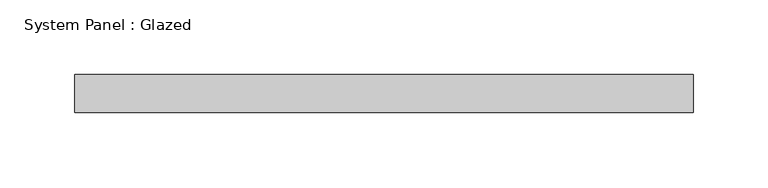
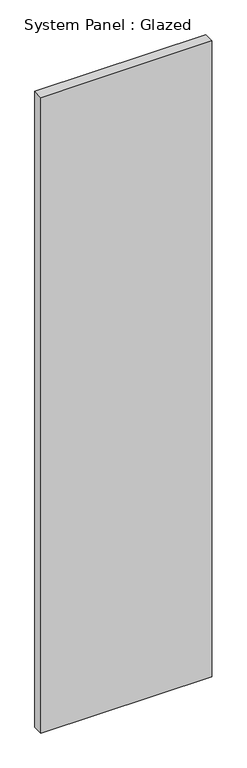
"""IFC4 building model written with IfcOpenShell, lengths in millimetres: plate geometry, System Panel : Glazed."""

from ifc_helpers import new_model, si_unit, origin, origin_with_axes, place, context, project, spatial, polyline, outline, extrude, source, transform, mapped, element, save


def system_panel_glazed_435c231b(model_context):
    return source(origin(), model_context, "Body", "SweptSolid", [
        extrude(outline(polyline([(206.375, 19.05), (-206.375, 19.05), (-206.375, 44.45), (206.375, 44.45), (206.375, 19.05)])), origin_with_axes(), (0.0, 0.0, 1.0), 1623.3622634),
    ])


if __name__ == "__main__":
    model = new_model("IFC4")
    model_context = context("Model", 3, world=origin())
    ifc_project = project(units=[si_unit("LENGTHUNIT", "METRE", prefix="MILLI")], contexts=[model_context])
    site = spatial("IfcSite", under=ifc_project)
    building = spatial("IfcBuilding", under=site)
    placement = place(None, origin())
    system_panel_glazed_shape = system_panel_glazed_435c231b(model_context)
    element("IfcPlate", 1, ObjectType="System Panel : Glazed", at=placement, inside=building, context=model_context, shape_type="MappedRepresentation", body=[
        mapped(system_panel_glazed_shape, transform((0.0, 0.0, 0.0), x_axis=(1.0, 0.0, 0.0), y_axis=(0.0, 1.0, 0.0), z_axis=(0.0, 0.0, 1.0))),
    ])
    save(model, "model.ifc")

# Revit data of these elements
# Type "System Panel : Glazed"
#   Construction Type Id = "GSP4R"
#   Analytic Construction = "1/8 in Pilkington single glazing"
#   Visual Light Transmittance = 0.9
#   Solar Heat Gain Coefficient = 0.86
#   Heat Transfer Coefficient (U) = 1.18115 BTU/(h·ft²·°F)
#   Define Thermal Properties by = 1
# Element 1 (IfcPlate, "System Panel : Glazed")
#   Materials on its faces: "Glass"
# Materials
#   "Glass": class "Glass", colour RGB 0 128 192, transparency 0.75, Description = "Soda Lime Glass", Cost = 0
